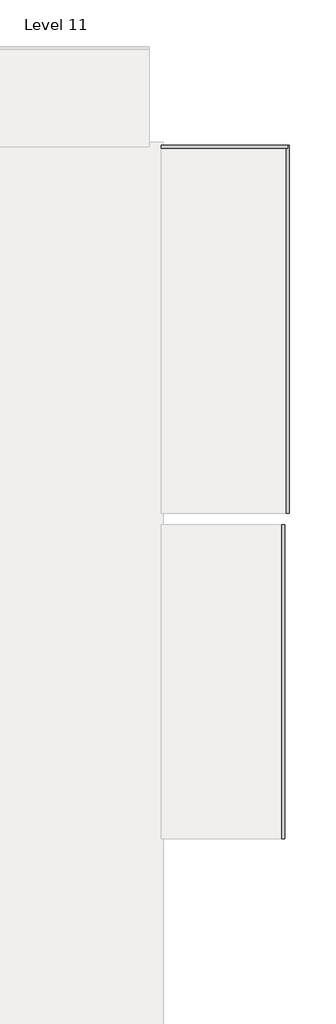
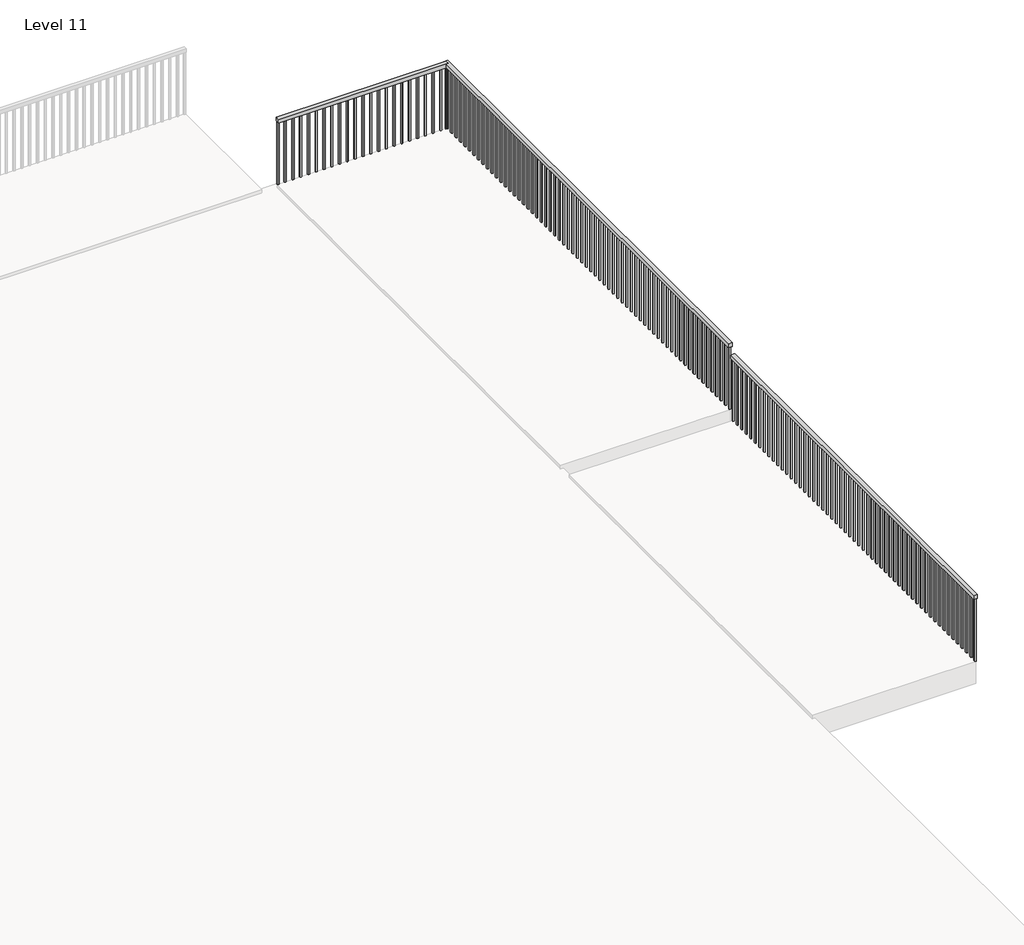
# One storey, part 4 of 5: 3 railings.
"""IFC4 building model written with IfcOpenShell, lengths in millimetres."""

from ifc_helpers import new_model, si_unit, frame, origin, place, context, project, spatial, polyline, outline, extrude, element, save

model = new_model("IFC4")

# Units and contexts
model_context = context("Model", 3, world=origin())
ifc_project = project(units=[si_unit("LENGTHUNIT", "METRE", prefix="MILLI")], contexts=[model_context])

# Site, building, storey
site = spatial("IfcSite", under=ifc_project)
building = spatial("IfcBuilding", under=site)
storey = spatial("IfcBuildingStorey", under=building, Name="Level 11", Elevation=15544.8)

# Railings
placement = place(None, origin())
element("IfcRailing", 1, ObjectType="Handrail - Rectangular", at=placement, inside=storey, context=model_context, shape_type="SweptSolid", body=[
    extrude(outline(polyline([(14106.5361222, 14743.2237525), (14106.5361222, 14794.0237525), (16321.4289933, 14794.0237525), (16321.4289933, 14743.2237525), (14106.5361222, 14743.2237525)])), frame((0.0, 0.0, 16408.4), z_axis=(0.0, 0.0, 1.0), x_axis=(1.0, 0.0, 0.0)), (0.0, 0.0, 1.0), 50.8),
    extrude(outline(polyline([(16230.6111222, 14759.0987525), (16230.6111222, 14778.1487525), (16249.6611222, 14778.1487525), (16249.6611222, 14759.0987525), (16230.6111222, 14759.0987525)])), frame((0.0, 0.0, 15544.8), z_axis=(0.0, 0.0, 1.0), x_axis=(1.0, 0.0, 0.0)), (0.0, 0.0, 1.0), 863.6),
    extrude(outline(polyline([(16129.0111222, 14759.0987525), (16129.0111222, 14778.1487525), (16148.0611222, 14778.1487525), (16148.0611222, 14759.0987525), (16129.0111222, 14759.0987525)])), frame((0.0, 0.0, 15544.8), z_axis=(0.0, 0.0, 1.0), x_axis=(1.0, 0.0, 0.0)), (0.0, 0.0, 1.0), 863.6),
    extrude(outline(polyline([(16027.4111222, 14759.0987525), (16027.4111222, 14778.1487525), (16046.4611222, 14778.1487525), (16046.4611222, 14759.0987525), (16027.4111222, 14759.0987525)])), frame((0.0, 0.0, 15544.8), z_axis=(0.0, 0.0, 1.0), x_axis=(1.0, 0.0, 0.0)), (0.0, 0.0, 1.0), 863.6),
    extrude(outline(polyline([(15925.8111222, 14759.0987525), (15925.8111222, 14778.1487525), (15944.8611222, 14778.1487525), (15944.8611222, 14759.0987525), (15925.8111222, 14759.0987525)])), frame((0.0, 0.0, 15544.8), z_axis=(0.0, 0.0, 1.0), x_axis=(1.0, 0.0, 0.0)), (0.0, 0.0, 1.0), 863.6),
    extrude(outline(polyline([(15824.2111222, 14759.0987525), (15824.2111222, 14778.1487525), (15843.2611222, 14778.1487525), (15843.2611222, 14759.0987525), (15824.2111222, 14759.0987525)])), frame((0.0, 0.0, 15544.8), z_axis=(0.0, 0.0, 1.0), x_axis=(1.0, 0.0, 0.0)), (0.0, 0.0, 1.0), 863.6),
    extrude(outline(polyline([(15722.6111222, 14759.0987525), (15722.6111222, 14778.1487525), (15741.6611222, 14778.1487525), (15741.6611222, 14759.0987525), (15722.6111222, 14759.0987525)])), frame((0.0, 0.0, 15544.8), z_axis=(0.0, 0.0, 1.0), x_axis=(1.0, 0.0, 0.0)), (0.0, 0.0, 1.0), 863.6),
    extrude(outline(polyline([(15621.0111222, 14759.0987525), (15621.0111222, 14778.1487525), (15640.0611222, 14778.1487525), (15640.0611222, 14759.0987525), (15621.0111222, 14759.0987525)])), frame((0.0, 0.0, 15544.8), z_axis=(0.0, 0.0, 1.0), x_axis=(1.0, 0.0, 0.0)), (0.0, 0.0, 1.0), 863.6),
    extrude(outline(polyline([(15519.4111222, 14759.0987525), (15519.4111222, 14778.1487525), (15538.4611222, 14778.1487525), (15538.4611222, 14759.0987525), (15519.4111222, 14759.0987525)])), frame((0.0, 0.0, 15544.8), z_axis=(0.0, 0.0, 1.0), x_axis=(1.0, 0.0, 0.0)), (0.0, 0.0, 1.0), 863.6),
    extrude(outline(polyline([(15417.8111222, 14759.0987525), (15417.8111222, 14778.1487525), (15436.8611222, 14778.1487525), (15436.8611222, 14759.0987525), (15417.8111222, 14759.0987525)])), frame((0.0, 0.0, 15544.8), z_axis=(0.0, 0.0, 1.0), x_axis=(1.0, 0.0, 0.0)), (0.0, 0.0, 1.0), 863.6),
    extrude(outline(polyline([(15316.2111222, 14759.0987525), (15316.2111222, 14778.1487525), (15335.2611222, 14778.1487525), (15335.2611222, 14759.0987525), (15316.2111222, 14759.0987525)])), frame((0.0, 0.0, 15544.8), z_axis=(0.0, 0.0, 1.0), x_axis=(1.0, 0.0, 0.0)), (0.0, 0.0, 1.0), 863.6),
    extrude(outline(polyline([(15214.6111222, 14759.0987525), (15214.6111222, 14778.1487525), (15233.6611222, 14778.1487525), (15233.6611222, 14759.0987525), (15214.6111222, 14759.0987525)])), frame((0.0, 0.0, 15544.8), z_axis=(0.0, 0.0, 1.0), x_axis=(1.0, 0.0, 0.0)), (0.0, 0.0, 1.0), 863.6),
    extrude(outline(polyline([(15113.0111222, 14759.0987525), (15113.0111222, 14778.1487525), (15132.0611222, 14778.1487525), (15132.0611222, 14759.0987525), (15113.0111222, 14759.0987525)])), frame((0.0, 0.0, 15544.8), z_axis=(0.0, 0.0, 1.0), x_axis=(1.0, 0.0, 0.0)), (0.0, 0.0, 1.0), 863.6),
    extrude(outline(polyline([(15011.4111222, 14759.0987525), (15011.4111222, 14778.1487525), (15030.4611222, 14778.1487525), (15030.4611222, 14759.0987525), (15011.4111222, 14759.0987525)])), frame((0.0, 0.0, 15544.8), z_axis=(0.0, 0.0, 1.0), x_axis=(1.0, 0.0, 0.0)), (0.0, 0.0, 1.0), 863.6),
    extrude(outline(polyline([(14909.8111222, 14759.0987525), (14909.8111222, 14778.1487525), (14928.8611222, 14778.1487525), (14928.8611222, 14759.0987525), (14909.8111222, 14759.0987525)])), frame((0.0, 0.0, 15544.8), z_axis=(0.0, 0.0, 1.0), x_axis=(1.0, 0.0, 0.0)), (0.0, 0.0, 1.0), 863.6),
    extrude(outline(polyline([(14808.2111222, 14759.0987525), (14808.2111222, 14778.1487525), (14827.2611222, 14778.1487525), (14827.2611222, 14759.0987525), (14808.2111222, 14759.0987525)])), frame((0.0, 0.0, 15544.8), z_axis=(0.0, 0.0, 1.0), x_axis=(1.0, 0.0, 0.0)), (0.0, 0.0, 1.0), 863.6),
    extrude(outline(polyline([(14706.6111222, 14759.0987525), (14706.6111222, 14778.1487525), (14725.6611222, 14778.1487525), (14725.6611222, 14759.0987525), (14706.6111222, 14759.0987525)])), frame((0.0, 0.0, 15544.8), z_axis=(0.0, 0.0, 1.0), x_axis=(1.0, 0.0, 0.0)), (0.0, 0.0, 1.0), 863.6),
    extrude(outline(polyline([(14605.0111222, 14759.0987525), (14605.0111222, 14778.1487525), (14624.0611222, 14778.1487525), (14624.0611222, 14759.0987525), (14605.0111222, 14759.0987525)])), frame((0.0, 0.0, 15544.8), z_axis=(0.0, 0.0, 1.0), x_axis=(1.0, 0.0, 0.0)), (0.0, 0.0, 1.0), 863.6),
    extrude(outline(polyline([(14503.4111222, 14759.0987525), (14503.4111222, 14778.1487525), (14522.4611222, 14778.1487525), (14522.4611222, 14759.0987525), (14503.4111222, 14759.0987525)])), frame((0.0, 0.0, 15544.8), z_axis=(0.0, 0.0, 1.0), x_axis=(1.0, 0.0, 0.0)), (0.0, 0.0, 1.0), 863.6),
    extrude(outline(polyline([(14401.8111222, 14759.0987525), (14401.8111222, 14778.1487525), (14420.8611222, 14778.1487525), (14420.8611222, 14759.0987525), (14401.8111222, 14759.0987525)])), frame((0.0, 0.0, 15544.8), z_axis=(0.0, 0.0, 1.0), x_axis=(1.0, 0.0, 0.0)), (0.0, 0.0, 1.0), 863.6),
    extrude(outline(polyline([(14300.2111222, 14759.0987525), (14300.2111222, 14778.1487525), (14319.2611222, 14778.1487525), (14319.2611222, 14759.0987525), (14300.2111222, 14759.0987525)])), frame((0.0, 0.0, 15544.8), z_axis=(0.0, 0.0, 1.0), x_axis=(1.0, 0.0, 0.0)), (0.0, 0.0, 1.0), 863.6),
    extrude(outline(polyline([(14198.6111222, 14759.0987525), (14198.6111222, 14778.1487525), (14217.6611222, 14778.1487525), (14217.6611222, 14759.0987525), (14198.6111222, 14759.0987525)])), frame((0.0, 0.0, 15544.8), z_axis=(0.0, 0.0, 1.0), x_axis=(1.0, 0.0, 0.0)), (0.0, 0.0, 1.0), 863.6),
    extrude(outline(polyline([(16302.3789933, 14759.0987525), (16302.3789933, 14778.1487525), (16321.4289933, 14778.1487525), (16321.4289933, 14759.0987525), (16302.3789933, 14759.0987525)])), frame((0.0, 0.0, 15544.8), z_axis=(0.0, 0.0, 1.0), x_axis=(1.0, 0.0, 0.0)), (0.0, 0.0, 1.0), 863.6),
    extrude(outline(polyline([(14106.5361222, 14759.0987525), (14106.5361222, 14778.1487525), (14125.5861222, 14778.1487525), (14125.5861222, 14759.0987525), (14106.5361222, 14759.0987525)])), frame((0.0, 0.0, 15544.8), z_axis=(0.0, 0.0, 1.0), x_axis=(1.0, 0.0, 0.0)), (0.0, 0.0, 1.0), 863.6),
])
element("IfcRailing", 2, ObjectType="Handrail - Rectangular", at=placement, inside=storey, context=model_context, shape_type="SweptSolid", body=[
    extrude(outline(polyline([(16346.8289933, 8367.8237525), (16296.0289933, 8367.8237525), (16296.0289933, 14794.0237525), (16346.8289933, 14794.0237525), (16346.8289933, 8367.8237525)])), frame((0.0, 0.0, 16408.4), z_axis=(0.0, 0.0, 1.0), x_axis=(1.0, 0.0, 0.0)), (0.0, 0.0, 1.0), 50.8),
    extrude(outline(polyline([(16330.9539933, 14759.0987525), (16311.9039933, 14759.0987525), (16311.9039933, 14778.1487525), (16330.9539933, 14778.1487525), (16330.9539933, 14759.0987525)])), frame((0.0, 0.0, 15544.8), z_axis=(0.0, 0.0, 1.0), x_axis=(1.0, 0.0, 0.0)), (0.0, 0.0, 1.0), 863.6),
    extrude(outline(polyline([(16330.9539933, 14657.4987525), (16311.9039933, 14657.4987525), (16311.9039933, 14676.5487525), (16330.9539933, 14676.5487525), (16330.9539933, 14657.4987525)])), frame((0.0, 0.0, 15544.8), z_axis=(0.0, 0.0, 1.0), x_axis=(1.0, 0.0, 0.0)), (0.0, 0.0, 1.0), 863.6),
    extrude(outline(polyline([(16330.9539933, 14555.8987525), (16311.9039933, 14555.8987525), (16311.9039933, 14574.9487525), (16330.9539933, 14574.9487525), (16330.9539933, 14555.8987525)])), frame((0.0, 0.0, 15544.8), z_axis=(0.0, 0.0, 1.0), x_axis=(1.0, 0.0, 0.0)), (0.0, 0.0, 1.0), 863.6),
    extrude(outline(polyline([(16330.9539933, 14454.2987525), (16311.9039933, 14454.2987525), (16311.9039933, 14473.3487525), (16330.9539933, 14473.3487525), (16330.9539933, 14454.2987525)])), frame((0.0, 0.0, 15544.8), z_axis=(0.0, 0.0, 1.0), x_axis=(1.0, 0.0, 0.0)), (0.0, 0.0, 1.0), 863.6),
    extrude(outline(polyline([(16330.9539933, 14352.6987525), (16311.9039933, 14352.6987525), (16311.9039933, 14371.7487525), (16330.9539933, 14371.7487525), (16330.9539933, 14352.6987525)])), frame((0.0, 0.0, 15544.8), z_axis=(0.0, 0.0, 1.0), x_axis=(1.0, 0.0, 0.0)), (0.0, 0.0, 1.0), 863.6),
    extrude(outline(polyline([(16330.9539933, 14251.0987525), (16311.9039933, 14251.0987525), (16311.9039933, 14270.1487525), (16330.9539933, 14270.1487525), (16330.9539933, 14251.0987525)])), frame((0.0, 0.0, 15544.8), z_axis=(0.0, 0.0, 1.0), x_axis=(1.0, 0.0, 0.0)), (0.0, 0.0, 1.0), 863.6),
    extrude(outline(polyline([(16330.9539933, 14149.4987525), (16311.9039933, 14149.4987525), (16311.9039933, 14168.5487525), (16330.9539933, 14168.5487525), (16330.9539933, 14149.4987525)])), frame((0.0, 0.0, 15544.8), z_axis=(0.0, 0.0, 1.0), x_axis=(1.0, 0.0, 0.0)), (0.0, 0.0, 1.0), 863.6),
    extrude(outline(polyline([(16330.9539933, 14047.8987525), (16311.9039933, 14047.8987525), (16311.9039933, 14066.9487525), (16330.9539933, 14066.9487525), (16330.9539933, 14047.8987525)])), frame((0.0, 0.0, 15544.8), z_axis=(0.0, 0.0, 1.0), x_axis=(1.0, 0.0, 0.0)), (0.0, 0.0, 1.0), 863.6),
    extrude(outline(polyline([(16330.9539933, 13946.2987525), (16311.9039933, 13946.2987525), (16311.9039933, 13965.3487525), (16330.9539933, 13965.3487525), (16330.9539933, 13946.2987525)])), frame((0.0, 0.0, 15544.8), z_axis=(0.0, 0.0, 1.0), x_axis=(1.0, 0.0, 0.0)), (0.0, 0.0, 1.0), 863.6),
    extrude(outline(polyline([(16330.9539933, 13844.6987525), (16311.9039933, 13844.6987525), (16311.9039933, 13863.7487525), (16330.9539933, 13863.7487525), (16330.9539933, 13844.6987525)])), frame((0.0, 0.0, 15544.8), z_axis=(0.0, 0.0, 1.0), x_axis=(1.0, 0.0, 0.0)), (0.0, 0.0, 1.0), 863.6),
    extrude(outline(polyline([(16330.9539933, 13743.0987525), (16311.9039933, 13743.0987525), (16311.9039933, 13762.1487525), (16330.9539933, 13762.1487525), (16330.9539933, 13743.0987525)])), frame((0.0, 0.0, 15544.8), z_axis=(0.0, 0.0, 1.0), x_axis=(1.0, 0.0, 0.0)), (0.0, 0.0, 1.0), 863.6),
    extrude(outline(polyline([(16330.9539933, 13641.4987525), (16311.9039933, 13641.4987525), (16311.9039933, 13660.5487525), (16330.9539933, 13660.5487525), (16330.9539933, 13641.4987525)])), frame((0.0, 0.0, 15544.8), z_axis=(0.0, 0.0, 1.0), x_axis=(1.0, 0.0, 0.0)), (0.0, 0.0, 1.0), 863.6),
    extrude(outline(polyline([(16330.9539933, 13539.8987525), (16311.9039933, 13539.8987525), (16311.9039933, 13558.9487525), (16330.9539933, 13558.9487525), (16330.9539933, 13539.8987525)])), frame((0.0, 0.0, 15544.8), z_axis=(0.0, 0.0, 1.0), x_axis=(1.0, 0.0, 0.0)), (0.0, 0.0, 1.0), 863.6),
    extrude(outline(polyline([(16330.9539933, 13438.2987525), (16311.9039933, 13438.2987525), (16311.9039933, 13457.3487525), (16330.9539933, 13457.3487525), (16330.9539933, 13438.2987525)])), frame((0.0, 0.0, 15544.8), z_axis=(0.0, 0.0, 1.0), x_axis=(1.0, 0.0, 0.0)), (0.0, 0.0, 1.0), 863.6),
    extrude(outline(polyline([(16330.9539933, 13336.6987525), (16311.9039933, 13336.6987525), (16311.9039933, 13355.7487525), (16330.9539933, 13355.7487525), (16330.9539933, 13336.6987525)])), frame((0.0, 0.0, 15544.8), z_axis=(0.0, 0.0, 1.0), x_axis=(1.0, 0.0, 0.0)), (0.0, 0.0, 1.0), 863.6),
    extrude(outline(polyline([(16330.9539933, 13235.0987525), (16311.9039933, 13235.0987525), (16311.9039933, 13254.1487525), (16330.9539933, 13254.1487525), (16330.9539933, 13235.0987525)])), frame((0.0, 0.0, 15544.8), z_axis=(0.0, 0.0, 1.0), x_axis=(1.0, 0.0, 0.0)), (0.0, 0.0, 1.0), 863.6),
    extrude(outline(polyline([(16330.9539933, 13133.4987525), (16311.9039933, 13133.4987525), (16311.9039933, 13152.5487525), (16330.9539933, 13152.5487525), (16330.9539933, 13133.4987525)])), frame((0.0, 0.0, 15544.8), z_axis=(0.0, 0.0, 1.0), x_axis=(1.0, 0.0, 0.0)), (0.0, 0.0, 1.0), 863.6),
    extrude(outline(polyline([(16330.9539933, 13031.8987525), (16311.9039933, 13031.8987525), (16311.9039933, 13050.9487525), (16330.9539933, 13050.9487525), (16330.9539933, 13031.8987525)])), frame((0.0, 0.0, 15544.8), z_axis=(0.0, 0.0, 1.0), x_axis=(1.0, 0.0, 0.0)), (0.0, 0.0, 1.0), 863.6),
    extrude(outline(polyline([(16330.9539933, 12930.2987525), (16311.9039933, 12930.2987525), (16311.9039933, 12949.3487525), (16330.9539933, 12949.3487525), (16330.9539933, 12930.2987525)])), frame((0.0, 0.0, 15544.8), z_axis=(0.0, 0.0, 1.0), x_axis=(1.0, 0.0, 0.0)), (0.0, 0.0, 1.0), 863.6),
    extrude(outline(polyline([(16330.9539933, 12828.6987525), (16311.9039933, 12828.6987525), (16311.9039933, 12847.7487525), (16330.9539933, 12847.7487525), (16330.9539933, 12828.6987525)])), frame((0.0, 0.0, 15544.8), z_axis=(0.0, 0.0, 1.0), x_axis=(1.0, 0.0, 0.0)), (0.0, 0.0, 1.0), 863.6),
    extrude(outline(polyline([(16330.9539933, 12727.0987525), (16311.9039933, 12727.0987525), (16311.9039933, 12746.1487525), (16330.9539933, 12746.1487525), (16330.9539933, 12727.0987525)])), frame((0.0, 0.0, 15544.8), z_axis=(0.0, 0.0, 1.0), x_axis=(1.0, 0.0, 0.0)), (0.0, 0.0, 1.0), 863.6),
    extrude(outline(polyline([(16330.9539933, 12625.4987525), (16311.9039933, 12625.4987525), (16311.9039933, 12644.5487525), (16330.9539933, 12644.5487525), (16330.9539933, 12625.4987525)])), frame((0.0, 0.0, 15544.8), z_axis=(0.0, 0.0, 1.0), x_axis=(1.0, 0.0, 0.0)), (0.0, 0.0, 1.0), 863.6),
    extrude(outline(polyline([(16330.9539933, 12523.8987525), (16311.9039933, 12523.8987525), (16311.9039933, 12542.9487525), (16330.9539933, 12542.9487525), (16330.9539933, 12523.8987525)])), frame((0.0, 0.0, 15544.8), z_axis=(0.0, 0.0, 1.0), x_axis=(1.0, 0.0, 0.0)), (0.0, 0.0, 1.0), 863.6),
    extrude(outline(polyline([(16330.9539933, 12422.2987525), (16311.9039933, 12422.2987525), (16311.9039933, 12441.3487525), (16330.9539933, 12441.3487525), (16330.9539933, 12422.2987525)])), frame((0.0, 0.0, 15544.8), z_axis=(0.0, 0.0, 1.0), x_axis=(1.0, 0.0, 0.0)), (0.0, 0.0, 1.0), 863.6),
    extrude(outline(polyline([(16330.9539933, 12320.6987525), (16311.9039933, 12320.6987525), (16311.9039933, 12339.7487525), (16330.9539933, 12339.7487525), (16330.9539933, 12320.6987525)])), frame((0.0, 0.0, 15544.8), z_axis=(0.0, 0.0, 1.0), x_axis=(1.0, 0.0, 0.0)), (0.0, 0.0, 1.0), 863.6),
    extrude(outline(polyline([(16330.9539933, 12219.0987525), (16311.9039933, 12219.0987525), (16311.9039933, 12238.1487525), (16330.9539933, 12238.1487525), (16330.9539933, 12219.0987525)])), frame((0.0, 0.0, 15544.8), z_axis=(0.0, 0.0, 1.0), x_axis=(1.0, 0.0, 0.0)), (0.0, 0.0, 1.0), 863.6),
    extrude(outline(polyline([(16330.9539933, 12117.4987525), (16311.9039933, 12117.4987525), (16311.9039933, 12136.5487525), (16330.9539933, 12136.5487525), (16330.9539933, 12117.4987525)])), frame((0.0, 0.0, 15544.8), z_axis=(0.0, 0.0, 1.0), x_axis=(1.0, 0.0, 0.0)), (0.0, 0.0, 1.0), 863.6),
    extrude(outline(polyline([(16330.9539933, 12015.8987525), (16311.9039933, 12015.8987525), (16311.9039933, 12034.9487525), (16330.9539933, 12034.9487525), (16330.9539933, 12015.8987525)])), frame((0.0, 0.0, 15544.8), z_axis=(0.0, 0.0, 1.0), x_axis=(1.0, 0.0, 0.0)), (0.0, 0.0, 1.0), 863.6),
    extrude(outline(polyline([(16330.9539933, 11914.2987525), (16311.9039933, 11914.2987525), (16311.9039933, 11933.3487525), (16330.9539933, 11933.3487525), (16330.9539933, 11914.2987525)])), frame((0.0, 0.0, 15544.8), z_axis=(0.0, 0.0, 1.0), x_axis=(1.0, 0.0, 0.0)), (0.0, 0.0, 1.0), 863.6),
    extrude(outline(polyline([(16330.9539933, 11812.6987525), (16311.9039933, 11812.6987525), (16311.9039933, 11831.7487525), (16330.9539933, 11831.7487525), (16330.9539933, 11812.6987525)])), frame((0.0, 0.0, 15544.8), z_axis=(0.0, 0.0, 1.0), x_axis=(1.0, 0.0, 0.0)), (0.0, 0.0, 1.0), 863.6),
    extrude(outline(polyline([(16330.9539933, 11711.0987525), (16311.9039933, 11711.0987525), (16311.9039933, 11730.1487525), (16330.9539933, 11730.1487525), (16330.9539933, 11711.0987525)])), frame((0.0, 0.0, 15544.8), z_axis=(0.0, 0.0, 1.0), x_axis=(1.0, 0.0, 0.0)), (0.0, 0.0, 1.0), 863.6),
    extrude(outline(polyline([(16330.9539933, 11609.4987525), (16311.9039933, 11609.4987525), (16311.9039933, 11628.5487525), (16330.9539933, 11628.5487525), (16330.9539933, 11609.4987525)])), frame((0.0, 0.0, 15544.8), z_axis=(0.0, 0.0, 1.0), x_axis=(1.0, 0.0, 0.0)), (0.0, 0.0, 1.0), 863.6),
    extrude(outline(polyline([(16330.9539933, 11507.8987525), (16311.9039933, 11507.8987525), (16311.9039933, 11526.9487525), (16330.9539933, 11526.9487525), (16330.9539933, 11507.8987525)])), frame((0.0, 0.0, 15544.8), z_axis=(0.0, 0.0, 1.0), x_axis=(1.0, 0.0, 0.0)), (0.0, 0.0, 1.0), 863.6),
    extrude(outline(polyline([(16330.9539933, 11406.2987525), (16311.9039933, 11406.2987525), (16311.9039933, 11425.3487525), (16330.9539933, 11425.3487525), (16330.9539933, 11406.2987525)])), frame((0.0, 0.0, 15544.8), z_axis=(0.0, 0.0, 1.0), x_axis=(1.0, 0.0, 0.0)), (0.0, 0.0, 1.0), 863.6),
    extrude(outline(polyline([(16330.9539933, 11304.6987525), (16311.9039933, 11304.6987525), (16311.9039933, 11323.7487525), (16330.9539933, 11323.7487525), (16330.9539933, 11304.6987525)])), frame((0.0, 0.0, 15544.8), z_axis=(0.0, 0.0, 1.0), x_axis=(1.0, 0.0, 0.0)), (0.0, 0.0, 1.0), 863.6),
    extrude(outline(polyline([(16330.9539933, 11203.0987525), (16311.9039933, 11203.0987525), (16311.9039933, 11222.1487525), (16330.9539933, 11222.1487525), (16330.9539933, 11203.0987525)])), frame((0.0, 0.0, 15544.8), z_axis=(0.0, 0.0, 1.0), x_axis=(1.0, 0.0, 0.0)), (0.0, 0.0, 1.0), 863.6),
    extrude(outline(polyline([(16330.9539933, 11101.4987525), (16311.9039933, 11101.4987525), (16311.9039933, 11120.5487525), (16330.9539933, 11120.5487525), (16330.9539933, 11101.4987525)])), frame((0.0, 0.0, 15544.8), z_axis=(0.0, 0.0, 1.0), x_axis=(1.0, 0.0, 0.0)), (0.0, 0.0, 1.0), 863.6),
    extrude(outline(polyline([(16330.9539933, 10999.8987525), (16311.9039933, 10999.8987525), (16311.9039933, 11018.9487525), (16330.9539933, 11018.9487525), (16330.9539933, 10999.8987525)])), frame((0.0, 0.0, 15544.8), z_axis=(0.0, 0.0, 1.0), x_axis=(1.0, 0.0, 0.0)), (0.0, 0.0, 1.0), 863.6),
    extrude(outline(polyline([(16330.9539933, 10898.2987525), (16311.9039933, 10898.2987525), (16311.9039933, 10917.3487525), (16330.9539933, 10917.3487525), (16330.9539933, 10898.2987525)])), frame((0.0, 0.0, 15544.8), z_axis=(0.0, 0.0, 1.0), x_axis=(1.0, 0.0, 0.0)), (0.0, 0.0, 1.0), 863.6),
    extrude(outline(polyline([(16330.9539933, 10796.6987525), (16311.9039933, 10796.6987525), (16311.9039933, 10815.7487525), (16330.9539933, 10815.7487525), (16330.9539933, 10796.6987525)])), frame((0.0, 0.0, 15544.8), z_axis=(0.0, 0.0, 1.0), x_axis=(1.0, 0.0, 0.0)), (0.0, 0.0, 1.0), 863.6),
    extrude(outline(polyline([(16330.9539933, 10695.0987525), (16311.9039933, 10695.0987525), (16311.9039933, 10714.1487525), (16330.9539933, 10714.1487525), (16330.9539933, 10695.0987525)])), frame((0.0, 0.0, 15544.8), z_axis=(0.0, 0.0, 1.0), x_axis=(1.0, 0.0, 0.0)), (0.0, 0.0, 1.0), 863.6),
    extrude(outline(polyline([(16330.9539933, 10593.4987525), (16311.9039933, 10593.4987525), (16311.9039933, 10612.5487525), (16330.9539933, 10612.5487525), (16330.9539933, 10593.4987525)])), frame((0.0, 0.0, 15544.8), z_axis=(0.0, 0.0, 1.0), x_axis=(1.0, 0.0, 0.0)), (0.0, 0.0, 1.0), 863.6),
    extrude(outline(polyline([(16330.9539933, 10491.8987525), (16311.9039933, 10491.8987525), (16311.9039933, 10510.9487525), (16330.9539933, 10510.9487525), (16330.9539933, 10491.8987525)])), frame((0.0, 0.0, 15544.8), z_axis=(0.0, 0.0, 1.0), x_axis=(1.0, 0.0, 0.0)), (0.0, 0.0, 1.0), 863.6),
    extrude(outline(polyline([(16330.9539933, 10390.2987525), (16311.9039933, 10390.2987525), (16311.9039933, 10409.3487525), (16330.9539933, 10409.3487525), (16330.9539933, 10390.2987525)])), frame((0.0, 0.0, 15544.8), z_axis=(0.0, 0.0, 1.0), x_axis=(1.0, 0.0, 0.0)), (0.0, 0.0, 1.0), 863.6),
    extrude(outline(polyline([(16330.9539933, 10288.6987525), (16311.9039933, 10288.6987525), (16311.9039933, 10307.7487525), (16330.9539933, 10307.7487525), (16330.9539933, 10288.6987525)])), frame((0.0, 0.0, 15544.8), z_axis=(0.0, 0.0, 1.0), x_axis=(1.0, 0.0, 0.0)), (0.0, 0.0, 1.0), 863.6),
    extrude(outline(polyline([(16330.9539933, 10187.0987525), (16311.9039933, 10187.0987525), (16311.9039933, 10206.1487525), (16330.9539933, 10206.1487525), (16330.9539933, 10187.0987525)])), frame((0.0, 0.0, 15544.8), z_axis=(0.0, 0.0, 1.0), x_axis=(1.0, 0.0, 0.0)), (0.0, 0.0, 1.0), 863.6),
    extrude(outline(polyline([(16330.9539933, 10085.4987525), (16311.9039933, 10085.4987525), (16311.9039933, 10104.5487525), (16330.9539933, 10104.5487525), (16330.9539933, 10085.4987525)])), frame((0.0, 0.0, 15544.8), z_axis=(0.0, 0.0, 1.0), x_axis=(1.0, 0.0, 0.0)), (0.0, 0.0, 1.0), 863.6),
    extrude(outline(polyline([(16330.9539933, 9983.8987525), (16311.9039933, 9983.8987525), (16311.9039933, 10002.9487525), (16330.9539933, 10002.9487525), (16330.9539933, 9983.8987525)])), frame((0.0, 0.0, 15544.8), z_axis=(0.0, 0.0, 1.0), x_axis=(1.0, 0.0, 0.0)), (0.0, 0.0, 1.0), 863.6),
    extrude(outline(polyline([(16330.9539933, 9882.2987525), (16311.9039933, 9882.2987525), (16311.9039933, 9901.3487525), (16330.9539933, 9901.3487525), (16330.9539933, 9882.2987525)])), frame((0.0, 0.0, 15544.8), z_axis=(0.0, 0.0, 1.0), x_axis=(1.0, 0.0, 0.0)), (0.0, 0.0, 1.0), 863.6),
    extrude(outline(polyline([(16330.9539933, 9780.6987525), (16311.9039933, 9780.6987525), (16311.9039933, 9799.7487525), (16330.9539933, 9799.7487525), (16330.9539933, 9780.6987525)])), frame((0.0, 0.0, 15544.8), z_axis=(0.0, 0.0, 1.0), x_axis=(1.0, 0.0, 0.0)), (0.0, 0.0, 1.0), 863.6),
    extrude(outline(polyline([(16330.9539933, 9679.0987525), (16311.9039933, 9679.0987525), (16311.9039933, 9698.1487525), (16330.9539933, 9698.1487525), (16330.9539933, 9679.0987525)])), frame((0.0, 0.0, 15544.8), z_axis=(0.0, 0.0, 1.0), x_axis=(1.0, 0.0, 0.0)), (0.0, 0.0, 1.0), 863.6),
    extrude(outline(polyline([(16330.9539933, 9577.4987525), (16311.9039933, 9577.4987525), (16311.9039933, 9596.5487525), (16330.9539933, 9596.5487525), (16330.9539933, 9577.4987525)])), frame((0.0, 0.0, 15544.8), z_axis=(0.0, 0.0, 1.0), x_axis=(1.0, 0.0, 0.0)), (0.0, 0.0, 1.0), 863.6),
    extrude(outline(polyline([(16330.9539933, 9475.8987525), (16311.9039933, 9475.8987525), (16311.9039933, 9494.9487525), (16330.9539933, 9494.9487525), (16330.9539933, 9475.8987525)])), frame((0.0, 0.0, 15544.8), z_axis=(0.0, 0.0, 1.0), x_axis=(1.0, 0.0, 0.0)), (0.0, 0.0, 1.0), 863.6),
    extrude(outline(polyline([(16330.9539933, 9374.2987525), (16311.9039933, 9374.2987525), (16311.9039933, 9393.3487525), (16330.9539933, 9393.3487525), (16330.9539933, 9374.2987525)])), frame((0.0, 0.0, 15544.8), z_axis=(0.0, 0.0, 1.0), x_axis=(1.0, 0.0, 0.0)), (0.0, 0.0, 1.0), 863.6),
    extrude(outline(polyline([(16330.9539933, 9272.6987525), (16311.9039933, 9272.6987525), (16311.9039933, 9291.7487525), (16330.9539933, 9291.7487525), (16330.9539933, 9272.6987525)])), frame((0.0, 0.0, 15544.8), z_axis=(0.0, 0.0, 1.0), x_axis=(1.0, 0.0, 0.0)), (0.0, 0.0, 1.0), 863.6),
    extrude(outline(polyline([(16330.9539933, 9171.0987525), (16311.9039933, 9171.0987525), (16311.9039933, 9190.1487525), (16330.9539933, 9190.1487525), (16330.9539933, 9171.0987525)])), frame((0.0, 0.0, 15544.8), z_axis=(0.0, 0.0, 1.0), x_axis=(1.0, 0.0, 0.0)), (0.0, 0.0, 1.0), 863.6),
    extrude(outline(polyline([(16330.9539933, 9069.4987525), (16311.9039933, 9069.4987525), (16311.9039933, 9088.5487525), (16330.9539933, 9088.5487525), (16330.9539933, 9069.4987525)])), frame((0.0, 0.0, 15544.8), z_axis=(0.0, 0.0, 1.0), x_axis=(1.0, 0.0, 0.0)), (0.0, 0.0, 1.0), 863.6),
    extrude(outline(polyline([(16330.9539933, 8967.8987525), (16311.9039933, 8967.8987525), (16311.9039933, 8986.9487525), (16330.9539933, 8986.9487525), (16330.9539933, 8967.8987525)])), frame((0.0, 0.0, 15544.8), z_axis=(0.0, 0.0, 1.0), x_axis=(1.0, 0.0, 0.0)), (0.0, 0.0, 1.0), 863.6),
    extrude(outline(polyline([(16330.9539933, 8866.2987525), (16311.9039933, 8866.2987525), (16311.9039933, 8885.3487525), (16330.9539933, 8885.3487525), (16330.9539933, 8866.2987525)])), frame((0.0, 0.0, 15544.8), z_axis=(0.0, 0.0, 1.0), x_axis=(1.0, 0.0, 0.0)), (0.0, 0.0, 1.0), 863.6),
    extrude(outline(polyline([(16330.9539933, 8764.6987525), (16311.9039933, 8764.6987525), (16311.9039933, 8783.7487525), (16330.9539933, 8783.7487525), (16330.9539933, 8764.6987525)])), frame((0.0, 0.0, 15544.8), z_axis=(0.0, 0.0, 1.0), x_axis=(1.0, 0.0, 0.0)), (0.0, 0.0, 1.0), 863.6),
    extrude(outline(polyline([(16330.9539933, 8663.0987525), (16311.9039933, 8663.0987525), (16311.9039933, 8682.1487525), (16330.9539933, 8682.1487525), (16330.9539933, 8663.0987525)])), frame((0.0, 0.0, 15544.8), z_axis=(0.0, 0.0, 1.0), x_axis=(1.0, 0.0, 0.0)), (0.0, 0.0, 1.0), 863.6),
    extrude(outline(polyline([(16330.9539933, 8561.4987525), (16311.9039933, 8561.4987525), (16311.9039933, 8580.5487525), (16330.9539933, 8580.5487525), (16330.9539933, 8561.4987525)])), frame((0.0, 0.0, 15544.8), z_axis=(0.0, 0.0, 1.0), x_axis=(1.0, 0.0, 0.0)), (0.0, 0.0, 1.0), 863.6),
    extrude(outline(polyline([(16330.9539933, 8459.8987525), (16311.9039933, 8459.8987525), (16311.9039933, 8478.9487525), (16330.9539933, 8478.9487525), (16330.9539933, 8459.8987525)])), frame((0.0, 0.0, 15544.8), z_axis=(0.0, 0.0, 1.0), x_axis=(1.0, 0.0, 0.0)), (0.0, 0.0, 1.0), 863.6),
    extrude(outline(polyline([(16330.9539933, 14774.9737525), (16311.9039933, 14774.9737525), (16311.9039933, 14794.0237525), (16330.9539933, 14794.0237525), (16330.9539933, 14774.9737525)])), frame((0.0, 0.0, 15544.8), z_axis=(0.0, 0.0, 1.0), x_axis=(1.0, 0.0, 0.0)), (0.0, 0.0, 1.0), 863.6),
    extrude(outline(polyline([(16330.9539933, 8367.8237525), (16311.9039933, 8367.8237525), (16311.9039933, 8386.8737525), (16330.9539933, 8386.8737525), (16330.9539933, 8367.8237525)])), frame((0.0, 0.0, 15544.8), z_axis=(0.0, 0.0, 1.0), x_axis=(1.0, 0.0, 0.0)), (0.0, 0.0, 1.0), 863.6),
])
element("IfcRailing", 3, ObjectType="Handrail - Rectangular", at=placement, inside=storey, context=model_context, shape_type="SweptSolid", body=[
    extrude(outline(polyline([(16214.7361222, 8164.6237525), (16265.5361222, 8164.6237525), (16265.5361222, 2678.2237525), (16214.7361222, 2678.2237525), (16214.7361222, 8164.6237525)])), frame((0.0, 0.0, 16408.4), z_axis=(0.0, 0.0, 1.0), x_axis=(1.0, 0.0, 0.0)), (0.0, 0.0, 1.0), 50.8),
    extrude(outline(polyline([(16230.6111222, 2789.3487525), (16249.6611222, 2789.3487525), (16249.6611222, 2770.2987525), (16230.6111222, 2770.2987525), (16230.6111222, 2789.3487525)])), frame((0.0, 0.0, 15544.8), z_axis=(0.0, 0.0, 1.0), x_axis=(1.0, 0.0, 0.0)), (0.0, 0.0, 1.0), 863.6),
    extrude(outline(polyline([(16230.6111222, 2890.9487525), (16249.6611222, 2890.9487525), (16249.6611222, 2871.8987525), (16230.6111222, 2871.8987525), (16230.6111222, 2890.9487525)])), frame((0.0, 0.0, 15544.8), z_axis=(0.0, 0.0, 1.0), x_axis=(1.0, 0.0, 0.0)), (0.0, 0.0, 1.0), 863.6),
    extrude(outline(polyline([(16230.6111222, 2992.5487525), (16249.6611222, 2992.5487525), (16249.6611222, 2973.4987525), (16230.6111222, 2973.4987525), (16230.6111222, 2992.5487525)])), frame((0.0, 0.0, 15544.8), z_axis=(0.0, 0.0, 1.0), x_axis=(1.0, 0.0, 0.0)), (0.0, 0.0, 1.0), 863.6),
    extrude(outline(polyline([(16230.6111222, 3094.1487525), (16249.6611222, 3094.1487525), (16249.6611222, 3075.0987525), (16230.6111222, 3075.0987525), (16230.6111222, 3094.1487525)])), frame((0.0, 0.0, 15544.8), z_axis=(0.0, 0.0, 1.0), x_axis=(1.0, 0.0, 0.0)), (0.0, 0.0, 1.0), 863.6),
    extrude(outline(polyline([(16230.6111222, 3195.7487525), (16249.6611222, 3195.7487525), (16249.6611222, 3176.6987525), (16230.6111222, 3176.6987525), (16230.6111222, 3195.7487525)])), frame((0.0, 0.0, 15544.8), z_axis=(0.0, 0.0, 1.0), x_axis=(1.0, 0.0, 0.0)), (0.0, 0.0, 1.0), 863.6),
    extrude(outline(polyline([(16230.6111222, 3297.3487525), (16249.6611222, 3297.3487525), (16249.6611222, 3278.2987525), (16230.6111222, 3278.2987525), (16230.6111222, 3297.3487525)])), frame((0.0, 0.0, 15544.8), z_axis=(0.0, 0.0, 1.0), x_axis=(1.0, 0.0, 0.0)), (0.0, 0.0, 1.0), 863.6),
    extrude(outline(polyline([(16230.6111222, 3398.9487525), (16249.6611222, 3398.9487525), (16249.6611222, 3379.8987525), (16230.6111222, 3379.8987525), (16230.6111222, 3398.9487525)])), frame((0.0, 0.0, 15544.8), z_axis=(0.0, 0.0, 1.0), x_axis=(1.0, 0.0, 0.0)), (0.0, 0.0, 1.0), 863.6),
    extrude(outline(polyline([(16230.6111222, 3500.5487525), (16249.6611222, 3500.5487525), (16249.6611222, 3481.4987525), (16230.6111222, 3481.4987525), (16230.6111222, 3500.5487525)])), frame((0.0, 0.0, 15544.8), z_axis=(0.0, 0.0, 1.0), x_axis=(1.0, 0.0, 0.0)), (0.0, 0.0, 1.0), 863.6),
    extrude(outline(polyline([(16230.6111222, 3602.1487525), (16249.6611222, 3602.1487525), (16249.6611222, 3583.0987525), (16230.6111222, 3583.0987525), (16230.6111222, 3602.1487525)])), frame((0.0, 0.0, 15544.8), z_axis=(0.0, 0.0, 1.0), x_axis=(1.0, 0.0, 0.0)), (0.0, 0.0, 1.0), 863.6),
    extrude(outline(polyline([(16230.6111222, 3703.7487525), (16249.6611222, 3703.7487525), (16249.6611222, 3684.6987525), (16230.6111222, 3684.6987525), (16230.6111222, 3703.7487525)])), frame((0.0, 0.0, 15544.8), z_axis=(0.0, 0.0, 1.0), x_axis=(1.0, 0.0, 0.0)), (0.0, 0.0, 1.0), 863.6),
    extrude(outline(polyline([(16230.6111222, 3805.3487525), (16249.6611222, 3805.3487525), (16249.6611222, 3786.2987525), (16230.6111222, 3786.2987525), (16230.6111222, 3805.3487525)])), frame((0.0, 0.0, 15544.8), z_axis=(0.0, 0.0, 1.0), x_axis=(1.0, 0.0, 0.0)), (0.0, 0.0, 1.0), 863.6),
    extrude(outline(polyline([(16230.6111222, 3906.9487525), (16249.6611222, 3906.9487525), (16249.6611222, 3887.8987525), (16230.6111222, 3887.8987525), (16230.6111222, 3906.9487525)])), frame((0.0, 0.0, 15544.8), z_axis=(0.0, 0.0, 1.0), x_axis=(1.0, 0.0, 0.0)), (0.0, 0.0, 1.0), 863.6),
    extrude(outline(polyline([(16230.6111222, 4008.5487525), (16249.6611222, 4008.5487525), (16249.6611222, 3989.4987525), (16230.6111222, 3989.4987525), (16230.6111222, 4008.5487525)])), frame((0.0, 0.0, 15544.8), z_axis=(0.0, 0.0, 1.0), x_axis=(1.0, 0.0, 0.0)), (0.0, 0.0, 1.0), 863.6),
    extrude(outline(polyline([(16230.6111222, 4110.1487525), (16249.6611222, 4110.1487525), (16249.6611222, 4091.0987525), (16230.6111222, 4091.0987525), (16230.6111222, 4110.1487525)])), frame((0.0, 0.0, 15544.8), z_axis=(0.0, 0.0, 1.0), x_axis=(1.0, 0.0, 0.0)), (0.0, 0.0, 1.0), 863.6),
    extrude(outline(polyline([(16230.6111222, 4211.7487525), (16249.6611222, 4211.7487525), (16249.6611222, 4192.6987525), (16230.6111222, 4192.6987525), (16230.6111222, 4211.7487525)])), frame((0.0, 0.0, 15544.8), z_axis=(0.0, 0.0, 1.0), x_axis=(1.0, 0.0, 0.0)), (0.0, 0.0, 1.0), 863.6),
    extrude(outline(polyline([(16230.6111222, 4313.3487525), (16249.6611222, 4313.3487525), (16249.6611222, 4294.2987525), (16230.6111222, 4294.2987525), (16230.6111222, 4313.3487525)])), frame((0.0, 0.0, 15544.8), z_axis=(0.0, 0.0, 1.0), x_axis=(1.0, 0.0, 0.0)), (0.0, 0.0, 1.0), 863.6),
    extrude(outline(polyline([(16230.6111222, 4414.9487525), (16249.6611222, 4414.9487525), (16249.6611222, 4395.8987525), (16230.6111222, 4395.8987525), (16230.6111222, 4414.9487525)])), frame((0.0, 0.0, 15544.8), z_axis=(0.0, 0.0, 1.0), x_axis=(1.0, 0.0, 0.0)), (0.0, 0.0, 1.0), 863.6),
    extrude(outline(polyline([(16230.6111222, 4516.5487525), (16249.6611222, 4516.5487525), (16249.6611222, 4497.4987525), (16230.6111222, 4497.4987525), (16230.6111222, 4516.5487525)])), frame((0.0, 0.0, 15544.8), z_axis=(0.0, 0.0, 1.0), x_axis=(1.0, 0.0, 0.0)), (0.0, 0.0, 1.0), 863.6),
    extrude(outline(polyline([(16230.6111222, 4618.1487525), (16249.6611222, 4618.1487525), (16249.6611222, 4599.0987525), (16230.6111222, 4599.0987525), (16230.6111222, 4618.1487525)])), frame((0.0, 0.0, 15544.8), z_axis=(0.0, 0.0, 1.0), x_axis=(1.0, 0.0, 0.0)), (0.0, 0.0, 1.0), 863.6),
    extrude(outline(polyline([(16230.6111222, 4719.7487525), (16249.6611222, 4719.7487525), (16249.6611222, 4700.6987525), (16230.6111222, 4700.6987525), (16230.6111222, 4719.7487525)])), frame((0.0, 0.0, 15544.8), z_axis=(0.0, 0.0, 1.0), x_axis=(1.0, 0.0, 0.0)), (0.0, 0.0, 1.0), 863.6),
    extrude(outline(polyline([(16230.6111222, 4821.3487525), (16249.6611222, 4821.3487525), (16249.6611222, 4802.2987525), (16230.6111222, 4802.2987525), (16230.6111222, 4821.3487525)])), frame((0.0, 0.0, 15544.8), z_axis=(0.0, 0.0, 1.0), x_axis=(1.0, 0.0, 0.0)), (0.0, 0.0, 1.0), 863.6),
    extrude(outline(polyline([(16230.6111222, 4922.9487525), (16249.6611222, 4922.9487525), (16249.6611222, 4903.8987525), (16230.6111222, 4903.8987525), (16230.6111222, 4922.9487525)])), frame((0.0, 0.0, 15544.8), z_axis=(0.0, 0.0, 1.0), x_axis=(1.0, 0.0, 0.0)), (0.0, 0.0, 1.0), 863.6),
    extrude(outline(polyline([(16230.6111222, 5024.5487525), (16249.6611222, 5024.5487525), (16249.6611222, 5005.4987525), (16230.6111222, 5005.4987525), (16230.6111222, 5024.5487525)])), frame((0.0, 0.0, 15544.8), z_axis=(0.0, 0.0, 1.0), x_axis=(1.0, 0.0, 0.0)), (0.0, 0.0, 1.0), 863.6),
    extrude(outline(polyline([(16230.6111222, 5126.1487525), (16249.6611222, 5126.1487525), (16249.6611222, 5107.0987525), (16230.6111222, 5107.0987525), (16230.6111222, 5126.1487525)])), frame((0.0, 0.0, 15544.8), z_axis=(0.0, 0.0, 1.0), x_axis=(1.0, 0.0, 0.0)), (0.0, 0.0, 1.0), 863.6),
    extrude(outline(polyline([(16230.6111222, 5227.7487525), (16249.6611222, 5227.7487525), (16249.6611222, 5208.6987525), (16230.6111222, 5208.6987525), (16230.6111222, 5227.7487525)])), frame((0.0, 0.0, 15544.8), z_axis=(0.0, 0.0, 1.0), x_axis=(1.0, 0.0, 0.0)), (0.0, 0.0, 1.0), 863.6),
    extrude(outline(polyline([(16230.6111222, 5329.3487525), (16249.6611222, 5329.3487525), (16249.6611222, 5310.2987525), (16230.6111222, 5310.2987525), (16230.6111222, 5329.3487525)])), frame((0.0, 0.0, 15544.8), z_axis=(0.0, 0.0, 1.0), x_axis=(1.0, 0.0, 0.0)), (0.0, 0.0, 1.0), 863.6),
    extrude(outline(polyline([(16230.6111222, 5430.9487525), (16249.6611222, 5430.9487525), (16249.6611222, 5411.8987525), (16230.6111222, 5411.8987525), (16230.6111222, 5430.9487525)])), frame((0.0, 0.0, 15544.8), z_axis=(0.0, 0.0, 1.0), x_axis=(1.0, 0.0, 0.0)), (0.0, 0.0, 1.0), 863.6),
    extrude(outline(polyline([(16230.6111222, 5532.5487525), (16249.6611222, 5532.5487525), (16249.6611222, 5513.4987525), (16230.6111222, 5513.4987525), (16230.6111222, 5532.5487525)])), frame((0.0, 0.0, 15544.8), z_axis=(0.0, 0.0, 1.0), x_axis=(1.0, 0.0, 0.0)), (0.0, 0.0, 1.0), 863.6),
    extrude(outline(polyline([(16230.6111222, 5634.1487525), (16249.6611222, 5634.1487525), (16249.6611222, 5615.0987525), (16230.6111222, 5615.0987525), (16230.6111222, 5634.1487525)])), frame((0.0, 0.0, 15544.8), z_axis=(0.0, 0.0, 1.0), x_axis=(1.0, 0.0, 0.0)), (0.0, 0.0, 1.0), 863.6),
    extrude(outline(polyline([(16230.6111222, 5735.7487525), (16249.6611222, 5735.7487525), (16249.6611222, 5716.6987525), (16230.6111222, 5716.6987525), (16230.6111222, 5735.7487525)])), frame((0.0, 0.0, 15544.8), z_axis=(0.0, 0.0, 1.0), x_axis=(1.0, 0.0, 0.0)), (0.0, 0.0, 1.0), 863.6),
    extrude(outline(polyline([(16230.6111222, 5837.3487525), (16249.6611222, 5837.3487525), (16249.6611222, 5818.2987525), (16230.6111222, 5818.2987525), (16230.6111222, 5837.3487525)])), frame((0.0, 0.0, 15544.8), z_axis=(0.0, 0.0, 1.0), x_axis=(1.0, 0.0, 0.0)), (0.0, 0.0, 1.0), 863.6),
    extrude(outline(polyline([(16230.6111222, 5938.9487525), (16249.6611222, 5938.9487525), (16249.6611222, 5919.8987525), (16230.6111222, 5919.8987525), (16230.6111222, 5938.9487525)])), frame((0.0, 0.0, 15544.8), z_axis=(0.0, 0.0, 1.0), x_axis=(1.0, 0.0, 0.0)), (0.0, 0.0, 1.0), 863.6),
    extrude(outline(polyline([(16230.6111222, 6040.5487525), (16249.6611222, 6040.5487525), (16249.6611222, 6021.4987525), (16230.6111222, 6021.4987525), (16230.6111222, 6040.5487525)])), frame((0.0, 0.0, 15544.8), z_axis=(0.0, 0.0, 1.0), x_axis=(1.0, 0.0, 0.0)), (0.0, 0.0, 1.0), 863.6),
    extrude(outline(polyline([(16230.6111222, 6142.1487525), (16249.6611222, 6142.1487525), (16249.6611222, 6123.0987525), (16230.6111222, 6123.0987525), (16230.6111222, 6142.1487525)])), frame((0.0, 0.0, 15544.8), z_axis=(0.0, 0.0, 1.0), x_axis=(1.0, 0.0, 0.0)), (0.0, 0.0, 1.0), 863.6),
    extrude(outline(polyline([(16230.6111222, 6243.7487525), (16249.6611222, 6243.7487525), (16249.6611222, 6224.6987525), (16230.6111222, 6224.6987525), (16230.6111222, 6243.7487525)])), frame((0.0, 0.0, 15544.8), z_axis=(0.0, 0.0, 1.0), x_axis=(1.0, 0.0, 0.0)), (0.0, 0.0, 1.0), 863.6),
    extrude(outline(polyline([(16230.6111222, 6345.3487525), (16249.6611222, 6345.3487525), (16249.6611222, 6326.2987525), (16230.6111222, 6326.2987525), (16230.6111222, 6345.3487525)])), frame((0.0, 0.0, 15544.8), z_axis=(0.0, 0.0, 1.0), x_axis=(1.0, 0.0, 0.0)), (0.0, 0.0, 1.0), 863.6),
    extrude(outline(polyline([(16230.6111222, 6446.9487525), (16249.6611222, 6446.9487525), (16249.6611222, 6427.8987525), (16230.6111222, 6427.8987525), (16230.6111222, 6446.9487525)])), frame((0.0, 0.0, 15544.8), z_axis=(0.0, 0.0, 1.0), x_axis=(1.0, 0.0, 0.0)), (0.0, 0.0, 1.0), 863.6),
    extrude(outline(polyline([(16230.6111222, 6548.5487525), (16249.6611222, 6548.5487525), (16249.6611222, 6529.4987525), (16230.6111222, 6529.4987525), (16230.6111222, 6548.5487525)])), frame((0.0, 0.0, 15544.8), z_axis=(0.0, 0.0, 1.0), x_axis=(1.0, 0.0, 0.0)), (0.0, 0.0, 1.0), 863.6),
    extrude(outline(polyline([(16230.6111222, 6650.1487525), (16249.6611222, 6650.1487525), (16249.6611222, 6631.0987525), (16230.6111222, 6631.0987525), (16230.6111222, 6650.1487525)])), frame((0.0, 0.0, 15544.8), z_axis=(0.0, 0.0, 1.0), x_axis=(1.0, 0.0, 0.0)), (0.0, 0.0, 1.0), 863.6),
    extrude(outline(polyline([(16230.6111222, 6751.7487525), (16249.6611222, 6751.7487525), (16249.6611222, 6732.6987525), (16230.6111222, 6732.6987525), (16230.6111222, 6751.7487525)])), frame((0.0, 0.0, 15544.8), z_axis=(0.0, 0.0, 1.0), x_axis=(1.0, 0.0, 0.0)), (0.0, 0.0, 1.0), 863.6),
    extrude(outline(polyline([(16230.6111222, 6853.3487525), (16249.6611222, 6853.3487525), (16249.6611222, 6834.2987525), (16230.6111222, 6834.2987525), (16230.6111222, 6853.3487525)])), frame((0.0, 0.0, 15544.8), z_axis=(0.0, 0.0, 1.0), x_axis=(1.0, 0.0, 0.0)), (0.0, 0.0, 1.0), 863.6),
    extrude(outline(polyline([(16230.6111222, 6954.9487525), (16249.6611222, 6954.9487525), (16249.6611222, 6935.8987525), (16230.6111222, 6935.8987525), (16230.6111222, 6954.9487525)])), frame((0.0, 0.0, 15544.8), z_axis=(0.0, 0.0, 1.0), x_axis=(1.0, 0.0, 0.0)), (0.0, 0.0, 1.0), 863.6),
    extrude(outline(polyline([(16230.6111222, 7056.5487525), (16249.6611222, 7056.5487525), (16249.6611222, 7037.4987525), (16230.6111222, 7037.4987525), (16230.6111222, 7056.5487525)])), frame((0.0, 0.0, 15544.8), z_axis=(0.0, 0.0, 1.0), x_axis=(1.0, 0.0, 0.0)), (0.0, 0.0, 1.0), 863.6),
    extrude(outline(polyline([(16230.6111222, 7158.1487525), (16249.6611222, 7158.1487525), (16249.6611222, 7139.0987525), (16230.6111222, 7139.0987525), (16230.6111222, 7158.1487525)])), frame((0.0, 0.0, 15544.8), z_axis=(0.0, 0.0, 1.0), x_axis=(1.0, 0.0, 0.0)), (0.0, 0.0, 1.0), 863.6),
    extrude(outline(polyline([(16230.6111222, 7259.7487525), (16249.6611222, 7259.7487525), (16249.6611222, 7240.6987525), (16230.6111222, 7240.6987525), (16230.6111222, 7259.7487525)])), frame((0.0, 0.0, 15544.8), z_axis=(0.0, 0.0, 1.0), x_axis=(1.0, 0.0, 0.0)), (0.0, 0.0, 1.0), 863.6),
    extrude(outline(polyline([(16230.6111222, 7361.3487525), (16249.6611222, 7361.3487525), (16249.6611222, 7342.2987525), (16230.6111222, 7342.2987525), (16230.6111222, 7361.3487525)])), frame((0.0, 0.0, 15544.8), z_axis=(0.0, 0.0, 1.0), x_axis=(1.0, 0.0, 0.0)), (0.0, 0.0, 1.0), 863.6),
    extrude(outline(polyline([(16230.6111222, 7462.9487525), (16249.6611222, 7462.9487525), (16249.6611222, 7443.8987525), (16230.6111222, 7443.8987525), (16230.6111222, 7462.9487525)])), frame((0.0, 0.0, 15544.8), z_axis=(0.0, 0.0, 1.0), x_axis=(1.0, 0.0, 0.0)), (0.0, 0.0, 1.0), 863.6),
    extrude(outline(polyline([(16230.6111222, 7564.5487525), (16249.6611222, 7564.5487525), (16249.6611222, 7545.4987525), (16230.6111222, 7545.4987525), (16230.6111222, 7564.5487525)])), frame((0.0, 0.0, 15544.8), z_axis=(0.0, 0.0, 1.0), x_axis=(1.0, 0.0, 0.0)), (0.0, 0.0, 1.0), 863.6),
    extrude(outline(polyline([(16230.6111222, 7666.1487525), (16249.6611222, 7666.1487525), (16249.6611222, 7647.0987525), (16230.6111222, 7647.0987525), (16230.6111222, 7666.1487525)])), frame((0.0, 0.0, 15544.8), z_axis=(0.0, 0.0, 1.0), x_axis=(1.0, 0.0, 0.0)), (0.0, 0.0, 1.0), 863.6),
    extrude(outline(polyline([(16230.6111222, 7767.7487525), (16249.6611222, 7767.7487525), (16249.6611222, 7748.6987525), (16230.6111222, 7748.6987525), (16230.6111222, 7767.7487525)])), frame((0.0, 0.0, 15544.8), z_axis=(0.0, 0.0, 1.0), x_axis=(1.0, 0.0, 0.0)), (0.0, 0.0, 1.0), 863.6),
    extrude(outline(polyline([(16230.6111222, 7869.3487525), (16249.6611222, 7869.3487525), (16249.6611222, 7850.2987525), (16230.6111222, 7850.2987525), (16230.6111222, 7869.3487525)])), frame((0.0, 0.0, 15544.8), z_axis=(0.0, 0.0, 1.0), x_axis=(1.0, 0.0, 0.0)), (0.0, 0.0, 1.0), 863.6),
    extrude(outline(polyline([(16230.6111222, 7970.9487525), (16249.6611222, 7970.9487525), (16249.6611222, 7951.8987525), (16230.6111222, 7951.8987525), (16230.6111222, 7970.9487525)])), frame((0.0, 0.0, 15544.8), z_axis=(0.0, 0.0, 1.0), x_axis=(1.0, 0.0, 0.0)), (0.0, 0.0, 1.0), 863.6),
    extrude(outline(polyline([(16230.6111222, 8072.5487525), (16249.6611222, 8072.5487525), (16249.6611222, 8053.4987525), (16230.6111222, 8053.4987525), (16230.6111222, 8072.5487525)])), frame((0.0, 0.0, 15544.8), z_axis=(0.0, 0.0, 1.0), x_axis=(1.0, 0.0, 0.0)), (0.0, 0.0, 1.0), 863.6),
    extrude(outline(polyline([(16230.6111222, 2697.2737525), (16249.6611222, 2697.2737525), (16249.6611222, 2678.2237525), (16230.6111222, 2678.2237525), (16230.6111222, 2697.2737525)])), frame((0.0, 0.0, 15544.8), z_axis=(0.0, 0.0, 1.0), x_axis=(1.0, 0.0, 0.0)), (0.0, 0.0, 1.0), 863.6),
    extrude(outline(polyline([(16230.6111222, 8164.6237525), (16249.6611222, 8164.6237525), (16249.6611222, 8145.5737525), (16230.6111222, 8145.5737525), (16230.6111222, 8164.6237525)])), frame((0.0, 0.0, 15544.8), z_axis=(0.0, 0.0, 1.0), x_axis=(1.0, 0.0, 0.0)), (0.0, 0.0, 1.0), 863.6),
])

save(model, "model.ifc")

# Revit data of these elements
# Type "Handrail - Rectangular"
#   Assembly Code = "C2010400"
#   built-in parameter 1008612 = 0.0416667 (stored number, unit not read)
#   built-in parameter 1008611 = 0.0416667 (stored number, unit not read)
#   built-in parameter 1008609 = 0.333333 (stored number, unit not read)
#   built-in parameter 1008604 = 0.166667 (stored number, unit not read)
#   built-in parameter 1008603 = 0.166667 (stored number, unit not read)
#   Railing Height = 3' - 0"
#   built-in parameter 1008630 = 2
#   built-in parameter 1008610 = 2
#   built-in parameter 1008618 = Baluster - Square : 3/4"
# Elements 1, 2, 3 (IfcRailing, "Handrail - Rectangular")
#   Phase Created = New Construction
